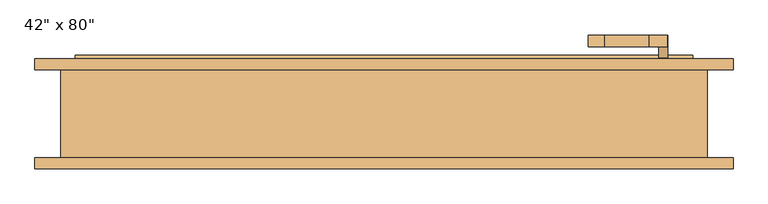
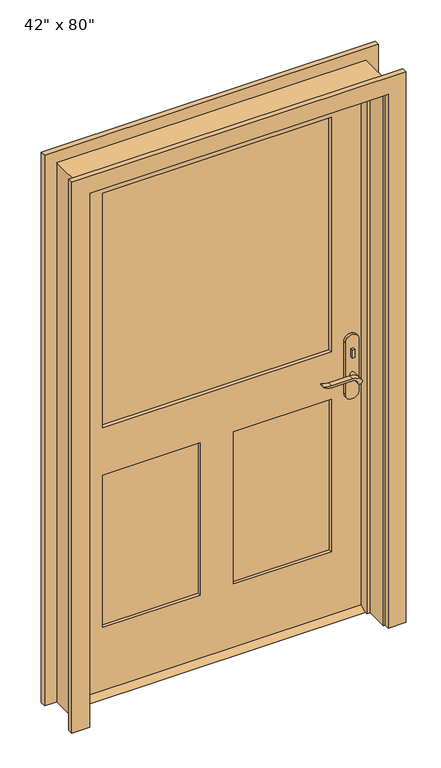
"""IFC4 building model written with IfcOpenShell, lengths in millimetres: door geometry."""

from ifc_helpers import new_model, si_unit, point, frame, frame_2d, origin, place, context, project, spatial, polyline, circle_curve, trimmed, segment, composite_curve, outline, extrude, faceted_brep, source, transform, mapped, element, save


def door_527a36f8(model_context):
    return source(origin(), model_context, "Body", "SolidModel", [
        extrude(outline(polyline([(38.1, 12.7), (73.025, 12.7), (98.425, 0.0), (12.7, 0.0), (38.1, 12.7)])), frame((-533.4, 0.0, 0.0), z_axis=(1.0, 0.0, 0.0), x_axis=(0.0, 1.0, 0.0)), (0.0, 0.0, 1.0), 1066.8),
        extrude(outline(polyline([(487.6, 18.1), (477.6, 18.1), (477.6, 28.1), (487.6, 28.1), (487.6, 18.1)])), frame((0.0, 0.0, 981.9), z_axis=(0.0, 0.0, 1.0), x_axis=(1.0, 0.0, 0.0)), (0.0, 0.0, 1.0), 30.0),
        extrude(outline(composite_curve([segment(trimmed(circle_curve(frame_2d((996.9, 482.6)), 8.0), [point((996.9, 474.6))], [point((996.9, 490.6))], False, "CARTESIAN"), True, "CONTINUOUS"), segment(trimmed(circle_curve(frame_2d((996.9, 482.6)), 8.0), [point((996.9, 490.6))], [point((996.9, 474.6))], False, "CARTESIAN"), True, "CONTINUOUS")], self_intersect=False)), frame((0.0, 83.025, 0.0), z_axis=(0.0, 1.0, 0.0), x_axis=(0.0, 0.0, 1.0)), (0.0, 0.0, 1.0), 10.0),
        extrude(outline(composite_curve([segment(trimmed(circle_curve(frame_2d((897.1555521, 458.9324871)), 37.2832219), [point((919.0523287, 489.1081363))], [point((934.4, 457.2325667))], False, "CARTESIAN"), True, "CONTINUOUS"), segment(polyline([(934.4, 457.2325667), (934.4, 380.9564091)]), True, "CONTINUOUS"), segment(trimmed(circle_curve(frame_2d((1017.6850638, 381.0227909)), 83.2850902), [point((934.4, 380.9564091))], [point((939.4, 352.6))], True, "CARTESIAN"), True, "CONTINUOUS"), segment(polyline([(939.4, 352.6), (936.6135558, 352.6)]), True, "CONTINUOUS"), segment(trimmed(circle_curve(frame_2d((986.6709207, 384.5396612)), 59.3791355), [point((936.6135558, 352.6))], [point((927.4, 380.9564091))], False, "CARTESIAN"), True, "CONTINUOUS"), segment(polyline([(927.4, 380.9564091), (927.4, 457.2138099)]), True, "CONTINUOUS"), segment(trimmed(circle_curve(frame_2d((909.2738613, 457.2138099)), 18.1261387), [point((927.4, 457.2138099))], [point((914.4, 474.6))], True, "CARTESIAN"), True, "CONTINUOUS"), segment(trimmed(circle_curve(frame_2d((914.4, 482.6)), 8.0), [point((914.4, 474.6))], [point((919.0523287, 489.1081363))], False, "CARTESIAN"), True, "CONTINUOUS")], self_intersect=False)), frame((0.0, -21.9, 0.0), z_axis=(0.0, 1.0, 0.0), x_axis=(0.0, 0.0, 1.0)), (0.0, 0.0, 1.0), 20.0),
        extrude(outline(composite_curve([segment(trimmed(circle_curve(frame_2d((914.4, 482.6)), 8.0), [point((914.3999903, 474.6))], [point((919.0523287, 489.1081363))], False, "CARTESIAN"), True, "CONTINUOUS"), segment(trimmed(circle_curve(frame_2d((897.1555521, 458.9324871)), 37.2832219), [point((919.0523287, 489.1081363))], [point((934.4, 457.2325667))], False, "CARTESIAN"), True, "CONTINUOUS"), segment(polyline([(934.4, 457.2325667), (934.4, 380.9564091)]), True, "CONTINUOUS"), segment(trimmed(circle_curve(frame_2d((1017.6850638, 381.0227909)), 83.2850902), [point((934.4, 380.9564091))], [point((939.4, 352.6))], True, "CARTESIAN"), True, "CONTINUOUS"), segment(polyline([(939.4, 352.6), (936.6135558, 352.6)]), True, "CONTINUOUS"), segment(trimmed(circle_curve(frame_2d((986.6709207, 384.5396612)), 59.3791355), [point((936.6135558, 352.6))], [point((927.4, 380.9564091))], False, "CARTESIAN"), True, "CONTINUOUS"), segment(polyline([(927.4, 380.9564091), (927.4, 457.2138122)]), True, "CONTINUOUS"), segment(trimmed(circle_curve(frame_2d((909.2738682, 457.2138122)), 18.1261318), [point((927.4, 457.2138122))], [point((914.3999903, 474.6))], True, "CARTESIAN"), True, "CONTINUOUS")], self_intersect=False)), frame((0.0, 113.025, 0.0), z_axis=(0.0, 1.0, 0.0), x_axis=(0.0, 0.0, 1.0)), (0.0, 0.0, 1.0), 20.0),
        extrude(outline(composite_curve([segment(trimmed(circle_curve(frame_2d((914.4, 482.6)), 8.0), [point((914.4, 474.6))], [point((914.4, 490.6))], False, "CARTESIAN"), True, "CONTINUOUS"), segment(trimmed(circle_curve(frame_2d((914.4, 482.6)), 8.0), [point((914.4, 490.6))], [point((914.4, 474.6))], False, "CARTESIAN"), True, "CONTINUOUS")], self_intersect=False)), frame((0.0, -1.9, 0.0), z_axis=(0.0, 1.0, 0.0), x_axis=(0.0, 0.0, 1.0)), (0.0, 0.0, 1.0), 30.0),
        extrude(outline(composite_curve([segment(trimmed(circle_curve(frame_2d((914.4, 482.6)), 8.0), [point((914.4, 474.6))], [point((914.4, 490.6))], False, "CARTESIAN"), True, "CONTINUOUS"), segment(trimmed(circle_curve(frame_2d((914.4, 482.6)), 8.0), [point((914.4, 490.6))], [point((914.4, 474.6))], False, "CARTESIAN"), True, "CONTINUOUS")], self_intersect=False)), frame((0.0, 83.025, 0.0), z_axis=(0.0, 1.0, 0.0), x_axis=(0.0, 0.0, 1.0)), (0.0, 0.0, 1.0), 30.0),
        extrude(outline(composite_curve([segment(polyline([(844.4, 507.6), (1039.4, 507.6)]), True, "CONTINUOUS"), segment(trimmed(circle_curve(frame_2d((1039.4, 482.6)), 25.0), [point((1039.4, 507.6))], [point((1039.4, 457.6))], False, "CARTESIAN"), True, "CONTINUOUS"), segment(polyline([(1039.4, 457.6), (844.4, 457.6)]), True, "CONTINUOUS"), segment(trimmed(circle_curve(frame_2d((844.4, 482.6)), 25.0), [point((844.4, 457.6))], [point((844.4, 507.6))], False, "CARTESIAN"), True, "CONTINUOUS")], self_intersect=False)), frame((0.0, 28.1, 0.0), z_axis=(0.0, 1.0, 0.0), x_axis=(0.0, 0.0, 1.0)), (0.0, 0.0, 1.0), 10.0),
        extrude(outline(composite_curve([segment(polyline([(844.4, 507.6), (1039.4, 507.6)]), True, "CONTINUOUS"), segment(trimmed(circle_curve(frame_2d((1039.4, 482.6)), 25.0), [point((1039.4, 507.6))], [point((1039.4, 457.6))], False, "CARTESIAN"), True, "CONTINUOUS"), segment(polyline([(1039.4, 457.6), (844.4, 457.6)]), True, "CONTINUOUS"), segment(trimmed(circle_curve(frame_2d((844.4, 482.6)), 25.0), [point((844.4, 457.6))], [point((844.4, 507.6))], False, "CARTESIAN"), True, "CONTINUOUS")], self_intersect=False)), frame((0.0, 73.025, 0.0), z_axis=(0.0, 1.0, 0.0), x_axis=(0.0, 0.0, 1.0)), (0.0, 0.0, 1.0), 10.0),
        extrude(outline(polyline([(2032.0, -533.4), (12.7, -533.4), (12.7, 533.4), (2032.0, 533.4), (2032.0, -533.4)]), holes=[polyline([(1016.0, -412.75), (1911.35, -412.75), (1911.35, 412.75), (1016.0, 412.75), (1016.0, -412.75)]), polyline([(835.025, -60.325), (254.0, -60.325), (254.0, -412.75), (835.025, -412.75), (835.025, -60.325)]), polyline([(835.025, 412.75), (254.0, 412.75), (254.0, 60.325), (835.025, 60.325), (835.025, 412.75)])]), frame((0.0, 38.1, 0.0), z_axis=(0.0, 1.0, 0.0), x_axis=(0.0, 0.0, 1.0)), (0.0, 0.0, 1.0), 34.925),
        faceted_brep([(558.8, 73.025, 0.0), (558.8, -79.375, 0.0), (533.4, -79.375, 0.0), (533.4, 3.175, 0.0), (520.7, 3.175, 0.0), (520.7, 38.1, 0.0), (533.4, 38.1, 0.0), (533.4, 73.025, 0.0), (558.8, 73.025, 2057.4), (558.8, -79.375, 2057.4), (-558.8, -79.375, 2057.4), (-558.8, -79.375, 0.0), (-533.4, -79.375, 0.0), (-533.4, -79.375, 2032.0), (533.4, -79.375, 2032.0), (533.4, 3.175, 2032.0), (-533.4, 3.175, 2032.0), (-533.4, 3.175, 0.0), (-520.7, 3.175, 0.0), (-520.7, 3.175, 2019.3), (520.7, 3.175, 2019.3), (520.7, 38.1, 2019.3), (-520.7, 38.1, 2019.3), (-520.7, 38.1, 0.0), (-533.4, 38.1, 0.0), (-533.4, 38.1, 2032.0), (533.4, 38.1, 2032.0), (533.4, 73.025, 2032.0), (-533.4, 73.025, 2032.0), (-533.4, 73.025, 0.0), (-558.8, 73.025, 0.0), (-558.8, 73.025, 2057.4)], [[[0, 1, 2, 3, 4, 5, 6, 7]], [[1, 0, 8, 9]], [[2, 1, 9, 10, 11, 12, 13, 14]], [[3, 2, 14, 15]], [[4, 3, 15, 16, 17, 18, 19, 20]], [[5, 4, 20, 21]], [[6, 5, 21, 22, 23, 24, 25, 26]], [[7, 6, 26, 27]], [[0, 7, 27, 28, 29, 30, 31, 8]], [[9, 8, 31, 10]], [[15, 14, 13, 16]], [[21, 20, 19, 22]], [[27, 26, 25, 28]], [[30, 29, 24, 23, 18, 17, 12, 11]], [[10, 31, 30, 11]], [[16, 13, 12, 17]], [[22, 19, 18, 23]], [[28, 25, 24, 29]]]),
        extrude(outline(polyline([(-60.325, 49.7416667), (-412.75, 49.7416667), (-412.75, 61.3833333), (-60.325, 61.3833333), (-60.325, 49.7416667)])), frame((0.0, 0.0, 254.0), z_axis=(0.0, 0.0, 1.0), x_axis=(1.0, 0.0, 0.0)), (0.0, 0.0, 1.0), 581.025),
        extrude(outline(polyline([(412.75, 49.7416667), (60.325, 49.7416667), (60.325, 61.3833333), (412.75, 61.3833333), (412.75, 49.7416667)])), frame((0.0, 0.0, 254.0), z_axis=(0.0, 0.0, 1.0), x_axis=(1.0, 0.0, 0.0)), (0.0, 0.0, 1.0), 581.025),
        extrude(outline(polyline([(412.75, 52.07), (-412.75, 52.07), (-412.75, 59.055), (412.75, 59.055), (412.75, 52.07)])), frame((0.0, 0.0, 1016.0), z_axis=(0.0, 0.0, 1.0), x_axis=(1.0, 0.0, 0.0)), (0.0, 0.0, 1.0), 895.35),
        extrude(outline(polyline([(0.0, -603.25), (0.0, -539.75), (2038.35, -539.75), (2038.35, 539.75), (0.0, 539.75), (0.0, 603.25), (2101.85, 603.25), (2101.85, -603.25), (0.0, -603.25)])), frame((0.0, -98.425, 0.0), z_axis=(0.0, 1.0, 0.0), x_axis=(0.0, 0.0, 1.0)), (0.0, 0.0, 1.0), 19.05),
        extrude(outline(polyline([(0.0, -603.25), (0.0, -539.75), (2038.35, -539.75), (2038.35, 539.75), (0.0, 539.75), (0.0, 603.25), (2101.85, 603.25), (2101.85, -603.25), (0.0, -603.25)])), frame((0.0, 73.025, 0.0), z_axis=(0.0, 1.0, 0.0), x_axis=(0.0, 0.0, 1.0)), (0.0, 0.0, 1.0), 19.05),
    ])


if __name__ == "__main__":
    model = new_model("IFC4")
    model_context = context("Model", 3, world=origin())
    ifc_project = project(units=[si_unit("LENGTHUNIT", "METRE", prefix="MILLI")], contexts=[model_context])
    site = spatial("IfcSite", under=ifc_project)
    building = spatial("IfcBuilding", under=site)
    placement = place(None, origin())
    door_shape = door_527a36f8(model_context)
    element("IfcDoor", 1, ObjectType="42\" x 80\"", at=placement, inside=building, context=model_context, shape_type="MappedRepresentation", body=[
        mapped(door_shape, transform((0.0, 0.0, 0.0), x_axis=(1.0, 0.0, 0.0), y_axis=(0.0, 1.0, 0.0), z_axis=(0.0, 0.0, 1.0))),
    ])
    save(model, "model.ifc")

# Revit data of these elements
# Type "42\" x 80\""
#   Type Mark = "8"
#   Assembly Code = "B2030100"
#   Analytic Construction = "French door, wood frame with single glass"
#   Top Rail = 0' - 4 3/4"
#   Threshold Offset [instance default] = 0' - 0 1/2"
#   Thickness = 0' - 1 3/8"
#   Thermal Resistance (R) = 1.0696 (h·ft²·°F)/BTU
#   Swing Angle [instance default] = 90.00°
#   Stiles = 0' - 4 3/4"
#   Rough Width = 3' - 8"
#   Rough Height = 6' - 9"
#   Lock Rail = 0' - 7 1/8"
#   Height = 6' - 8"
#   Width = 3' - 6"
#   Heat Transfer Coefficient (U) = 0.9350 BTU/(h·ft²·°F)
#   Door Offset [instance default] = 0' - 0"
#   Bottom Rail = 0' - 9 1/2"
#   Threshold [instance default] = yes
#   Function = 1
#   Exterior Trim [instance default] = yes
#   Trim Material = Cherry
#   Threshold Material = Cherry
#   Panel Material = Cherry
#   Glazing = Glass
#   Frame Material = Cherry
#   Door Handle Material = Aluminum
#   Visual Light Transmittance = 0
#   Solar Heat Gain Coefficient = 0
#   Wall Closure = (empty or 0)
#   Construction Type = (empty or 0)
# Element 1 (IfcDoor, "42\" x 80\"")
#   Materials on its faces: "Cherry", "Aluminum", "Glass"
# Materials
#   "Cherry": class "Wood", colour RGB 226 177 128, transparency 0, Description = "Prunus Serotina", Cost = 0
#   "Glass": class "Glass", colour RGB 0 128 192, transparency 0.75, Description = "Soda Lime Glass", Cost = 0
#   "Aluminum": class "Metal", colour RGB 247 247 247, transparency 0, Description = "Aluminum 6061", Cost = 0
